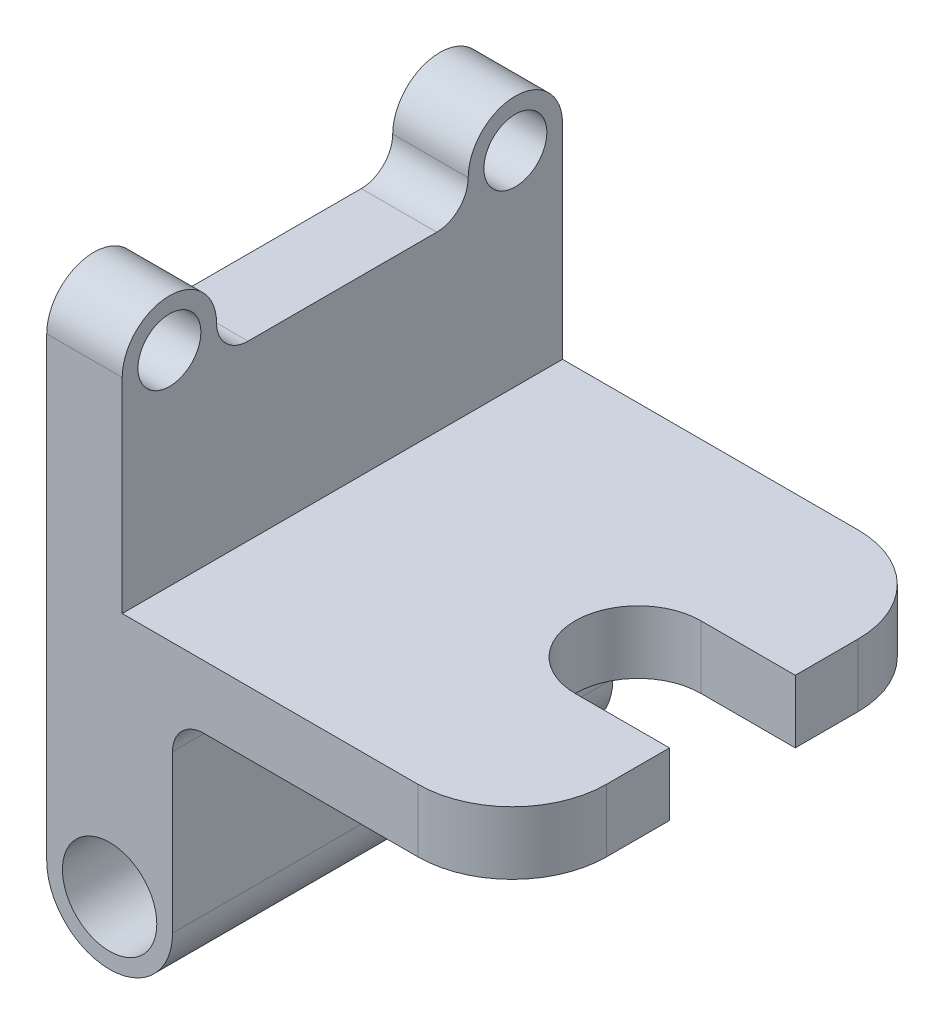
ISO-10303-21;
HEADER;
FILE_DESCRIPTION(('STEP AP214'),'2;1');
FILE_NAME('part.step','',(''),(''),'','','');
FILE_SCHEMA(('AUTOMOTIVE_DESIGN { 1 0 10303 214 1 1 1 1 }'));
ENDSEC;
DATA;
#1=APPLICATION_CONTEXT('core data for automotive mechanical design processes');
#2=APPLICATION_PROTOCOL_DEFINITION('international standard','automotive_design',2000,#1);
#3=PRODUCT_CONTEXT('',#1,'mechanical');
#4=PRODUCT('Part','Part','',(#3));
#5=PRODUCT_RELATED_PRODUCT_CATEGORY('part','',(#4));
#6=PRODUCT_DEFINITION_FORMATION('','',#4);
#7=PRODUCT_DEFINITION_CONTEXT('part definition',#1,'design');
#8=PRODUCT_DEFINITION('design','',#6,#7);
#9=PRODUCT_DEFINITION_SHAPE('','',#8);
#10=(LENGTH_UNIT() NAMED_UNIT(*) SI_UNIT(.MILLI.,.METRE.));
#11=(NAMED_UNIT(*) PLANE_ANGLE_UNIT() SI_UNIT($,.RADIAN.));
#12=(NAMED_UNIT(*) SI_UNIT($,.STERADIAN.) SOLID_ANGLE_UNIT());
#13=UNCERTAINTY_MEASURE_WITH_UNIT(LENGTH_MEASURE(1.E-05),#10,'distance_accuracy_value','');
#14=(GEOMETRIC_REPRESENTATION_CONTEXT(3) GLOBAL_UNCERTAINTY_ASSIGNED_CONTEXT((#13)) GLOBAL_UNIT_ASSIGNED_CONTEXT((#10,
#11,#12)) REPRESENTATION_CONTEXT('',''));
#15=CARTESIAN_POINT('',(0.,0.,0.));
#16=DIRECTION('',(0.,0.,1.));
#17=DIRECTION('',(1.,0.,0.));
#18=AXIS2_PLACEMENT_3D('',#15,#16,#17);
#19=CARTESIAN_POINT('',(0.,5.,35.));
#20=DIRECTION('',(0.,0.,-1.));
#21=DIRECTION('',(-1.,0.,0.));
#22=AXIS2_PLACEMENT_3D('',#19,#20,#21);
#23=PLANE('',#22);
#24=DIRECTION('',(0.,1.,0.));
#25=VECTOR('',#24,1.);
#26=CARTESIAN_POINT('',(-12.,-5.,35.));
#27=LINE('',#26,#25);
#28=CARTESIAN_POINT('',(-12.,-35.,35.));
#29=VERTEX_POINT('',#28);
#30=CARTESIAN_POINT('',(-12.,37.5,35.));
#31=VERTEX_POINT('',#30);
#32=EDGE_CURVE('E175',#29,#31,#27,.T.);
#33=ORIENTED_EDGE('',*,*,#32,.F.);
#34=CARTESIAN_POINT('',(-2.,-35.,35.));
#35=DIRECTION('',(0.,0.,1.));
#36=DIRECTION('',(1.,0.,0.));
#37=AXIS2_PLACEMENT_3D('',#34,#35,#36);
#38=CIRCLE('',#37,10.);
#39=CARTESIAN_POINT('',(8.,-35.,35.));
#40=VERTEX_POINT('',#39);
#41=EDGE_CURVE('E180',#29,#40,#38,.T.);
#42=ORIENTED_EDGE('',*,*,#41,.T.);
#43=DIRECTION('',(0.,1.,0.));
#44=VECTOR('',#43,1.);
#45=CARTESIAN_POINT('',(8.,-5.,35.));
#46=LINE('',#45,#44);
#47=CARTESIAN_POINT('',(8.,-10.,35.));
#48=VERTEX_POINT('',#47);
#49=EDGE_CURVE('E193',#40,#48,#46,.T.);
#50=ORIENTED_EDGE('',*,*,#49,.T.);
#51=CARTESIAN_POINT('',(13.,-10.,35.));
#52=DIRECTION('',(0.,0.,-1.));
#53=DIRECTION('',(-1.,0.,0.));
#54=AXIS2_PLACEMENT_3D('',#51,#52,#53);
#55=CIRCLE('',#54,5.);
#56=CARTESIAN_POINT('',(13.,-5.,35.));
#57=VERTEX_POINT('',#56);
#58=EDGE_CURVE('E11',#48,#57,#55,.T.);
#59=ORIENTED_EDGE('',*,*,#58,.T.);
#60=DIRECTION('',(1.,0.,0.));
#61=VECTOR('',#60,1.);
#62=CARTESIAN_POINT('',(0.,-5.,35.));
#63=LINE('',#62,#61);
#64=CARTESIAN_POINT('',(47.,-5.,35.));
#65=VERTEX_POINT('',#64);
#66=EDGE_CURVE('E246',#57,#65,#63,.T.);
#67=ORIENTED_EDGE('',*,*,#66,.T.);
#68=DIRECTION('',(0.,-1.,0.));
#69=VECTOR('',#68,1.);
#70=CARTESIAN_POINT('',(47.,5.,35.));
#71=LINE('',#70,#69);
#72=CARTESIAN_POINT('',(47.,5.,35.));
#73=VERTEX_POINT('',#72);
#74=EDGE_CURVE('E306',#73,#65,#71,.T.);
#75=ORIENTED_EDGE('',*,*,#74,.F.);
#76=DIRECTION('',(1.,0.,0.));
#77=VECTOR('',#76,1.);
#78=CARTESIAN_POINT('',(0.,5.,35.));
#79=LINE('',#78,#77);
#80=CARTESIAN_POINT('',(0.,5.,35.));
#81=VERTEX_POINT('',#80);
#82=EDGE_CURVE('E253',#81,#73,#79,.T.);
#83=ORIENTED_EDGE('',*,*,#82,.F.);
#84=DIRECTION('',(0.,1.,0.));
#85=VECTOR('',#84,1.);
#86=CARTESIAN_POINT('',(0.,5.,35.));
#87=LINE('',#86,#85);
#88=CARTESIAN_POINT('',(0.,37.5,35.));
#89=VERTEX_POINT('',#88);
#90=EDGE_CURVE('E214',#81,#89,#87,.T.);
#91=ORIENTED_EDGE('',*,*,#90,.T.);
#92=DIRECTION('',(1.,0.,0.));
#93=VECTOR('',#92,1.);
#94=CARTESIAN_POINT('',(-12.,37.5,35.));
#95=LINE('',#94,#93);
#96=EDGE_CURVE('E182',#31,#89,#95,.T.);
#97=ORIENTED_EDGE('',*,*,#96,.F.);
#98=EDGE_LOOP('',(#33,#42,#50,#59,#67,#75,#83,#91,#97));
#99=FACE_BOUND('',#98,.T.);
#100=CARTESIAN_POINT('',(-2.,-35.,35.));
#101=DIRECTION('',(0.,0.,1.));
#102=DIRECTION('',(1.,0.,0.));
#103=AXIS2_PLACEMENT_3D('',#100,#101,#102);
#104=CIRCLE('',#103,7.5);
#105=CARTESIAN_POINT('',(5.5,-35.,35.));
#106=VERTEX_POINT('',#105);
#107=EDGE_CURVE('E657',#106,#106,#104,.T.);
#108=ORIENTED_EDGE('',*,*,#107,.F.);
#109=EDGE_LOOP('',(#108));
#110=FACE_BOUND('',#109,.T.);
#111=ADVANCED_FACE('F44',(#99,#110),#23,.F.);
#112=CARTESIAN_POINT('',(47.,5.,20.));
#113=DIRECTION('',(0.,-1.,0.));
#114=DIRECTION('',(0.,0.,-1.));
#115=AXIS2_PLACEMENT_3D('',#112,#113,#114);
#116=CYLINDRICAL_SURFACE('',#115,15.);
#117=CARTESIAN_POINT('',(47.,-5.,20.));
#118=DIRECTION('',(0.,1.,0.));
#119=DIRECTION('',(0.,0.,1.));
#120=AXIS2_PLACEMENT_3D('',#117,#118,#119);
#121=CIRCLE('',#120,15.);
#122=CARTESIAN_POINT('',(62.,-5.,20.));
#123=VERTEX_POINT('',#122);
#124=EDGE_CURVE('E272',#65,#123,#121,.T.);
#125=ORIENTED_EDGE('',*,*,#124,.T.);
#126=DIRECTION('',(0.,-1.,0.));
#127=VECTOR('',#126,1.);
#128=CARTESIAN_POINT('',(62.,5.,20.));
#129=LINE('',#128,#127);
#130=CARTESIAN_POINT('',(62.,5.,20.));
#131=VERTEX_POINT('',#130);
#132=EDGE_CURVE('E302',#131,#123,#129,.T.);
#133=ORIENTED_EDGE('',*,*,#132,.F.);
#134=CARTESIAN_POINT('',(47.,5.,20.));
#135=DIRECTION('',(0.,1.,0.));
#136=DIRECTION('',(0.,0.,1.));
#137=AXIS2_PLACEMENT_3D('',#134,#135,#136);
#138=CIRCLE('',#137,15.);
#139=EDGE_CURVE('E255',#73,#131,#138,.T.);
#140=ORIENTED_EDGE('',*,*,#139,.F.);
#141=ORIENTED_EDGE('',*,*,#74,.T.);
#142=EDGE_LOOP('',(#125,#133,#140,#141));
#143=FACE_BOUND('',#142,.T.);
#144=ADVANCED_FACE('F371',(#143),#116,.T.);
#145=CARTESIAN_POINT('',(62.,5.,10.));
#146=DIRECTION('',(-1.,0.,0.));
#147=DIRECTION('',(0.,0.,1.));
#148=AXIS2_PLACEMENT_3D('',#145,#146,#147);
#149=PLANE('',#148);
#150=DIRECTION('',(0.,0.,-1.));
#151=VECTOR('',#150,1.);
#152=CARTESIAN_POINT('',(62.,-5.,10.));
#153=LINE('',#152,#151);
#154=CARTESIAN_POINT('',(62.,-5.,10.));
#155=VERTEX_POINT('',#154);
#156=EDGE_CURVE('E274',#123,#155,#153,.T.);
#157=ORIENTED_EDGE('',*,*,#156,.T.);
#158=DIRECTION('',(0.,-1.,0.));
#159=VECTOR('',#158,1.);
#160=CARTESIAN_POINT('',(62.,5.,10.));
#161=LINE('',#160,#159);
#162=CARTESIAN_POINT('',(62.,5.,10.));
#163=VERTEX_POINT('',#162);
#164=EDGE_CURVE('E301',#163,#155,#161,.T.);
#165=ORIENTED_EDGE('',*,*,#164,.F.);
#166=DIRECTION('',(0.,0.,-1.));
#167=VECTOR('',#166,1.);
#168=CARTESIAN_POINT('',(62.,5.,10.));
#169=LINE('',#168,#167);
#170=EDGE_CURVE('E258',#131,#163,#169,.T.);
#171=ORIENTED_EDGE('',*,*,#170,.F.);
#172=ORIENTED_EDGE('',*,*,#132,.T.);
#173=EDGE_LOOP('',(#157,#165,#171,#172));
#174=FACE_BOUND('',#173,.T.);
#175=ADVANCED_FACE('F370',(#174),#149,.F.);
#176=CARTESIAN_POINT('',(47.,5.,10.));
#177=DIRECTION('',(0.,0.,1.));
#178=DIRECTION('',(1.,0.,0.));
#179=AXIS2_PLACEMENT_3D('',#176,#177,#178);
#180=PLANE('',#179);
#181=DIRECTION('',(-1.,0.,0.));
#182=VECTOR('',#181,1.);
#183=CARTESIAN_POINT('',(47.,-5.,10.));
#184=LINE('',#183,#182);
#185=CARTESIAN_POINT('',(47.,-5.,10.));
#186=VERTEX_POINT('',#185);
#187=EDGE_CURVE('E280',#155,#186,#184,.T.);
#188=ORIENTED_EDGE('',*,*,#187,.T.);
#189=DIRECTION('',(0.,-1.,0.));
#190=VECTOR('',#189,1.);
#191=CARTESIAN_POINT('',(47.,5.,10.));
#192=LINE('',#191,#190);
#193=CARTESIAN_POINT('',(47.,5.,10.));
#194=VERTEX_POINT('',#193);
#195=EDGE_CURVE('E298',#194,#186,#192,.T.);
#196=ORIENTED_EDGE('',*,*,#195,.F.);
#197=DIRECTION('',(-1.,0.,0.));
#198=VECTOR('',#197,1.);
#199=CARTESIAN_POINT('',(47.,5.,10.));
#200=LINE('',#199,#198);
#201=EDGE_CURVE('E256',#163,#194,#200,.T.);
#202=ORIENTED_EDGE('',*,*,#201,.F.);
#203=ORIENTED_EDGE('',*,*,#164,.T.);
#204=EDGE_LOOP('',(#188,#196,#202,#203));
#205=FACE_BOUND('',#204,.T.);
#206=ADVANCED_FACE('F362',(#205),#180,.F.);
#207=CARTESIAN_POINT('',(47.,5.,0.));
#208=DIRECTION('',(0.,-1.,0.));
#209=DIRECTION('',(0.,0.,-1.));
#210=AXIS2_PLACEMENT_3D('',#207,#208,#209);
#211=CYLINDRICAL_SURFACE('',#210,10.);
#212=CARTESIAN_POINT('',(47.,-5.,0.));
#213=DIRECTION('',(0.,-1.,0.));
#214=DIRECTION('',(0.,0.,1.));
#215=AXIS2_PLACEMENT_3D('',#212,#213,#214);
#216=CIRCLE('',#215,10.);
#217=CARTESIAN_POINT('',(47.,-5.,-10.));
#218=VERTEX_POINT('',#217);
#219=EDGE_CURVE('E276',#186,#218,#216,.T.);
#220=ORIENTED_EDGE('',*,*,#219,.T.);
#221=DIRECTION('',(0.,-1.,0.));
#222=VECTOR('',#221,1.);
#223=CARTESIAN_POINT('',(47.,5.,-10.));
#224=LINE('',#223,#222);
#225=CARTESIAN_POINT('',(47.,5.,-10.));
#226=VERTEX_POINT('',#225);
#227=EDGE_CURVE('E296',#226,#218,#224,.T.);
#228=ORIENTED_EDGE('',*,*,#227,.F.);
#229=CARTESIAN_POINT('',(47.,5.,0.));
#230=DIRECTION('',(0.,-1.,0.));
#231=DIRECTION('',(0.,0.,1.));
#232=AXIS2_PLACEMENT_3D('',#229,#230,#231);
#233=CIRCLE('',#232,10.);
#234=EDGE_CURVE('E257',#194,#226,#233,.T.);
#235=ORIENTED_EDGE('',*,*,#234,.F.);
#236=ORIENTED_EDGE('',*,*,#195,.T.);
#237=EDGE_LOOP('',(#220,#228,#235,#236));
#238=FACE_BOUND('',#237,.T.);
#239=ADVANCED_FACE('F356',(#238),#211,.F.);
#240=CARTESIAN_POINT('',(47.,5.,-10.));
#241=DIRECTION('',(0.,0.,-1.));
#242=DIRECTION('',(-1.,0.,0.));
#243=AXIS2_PLACEMENT_3D('',#240,#241,#242);
#244=PLANE('',#243);
#245=DIRECTION('',(1.,0.,0.));
#246=VECTOR('',#245,1.);
#247=CARTESIAN_POINT('',(47.,-5.,-10.));
#248=LINE('',#247,#246);
#249=CARTESIAN_POINT('',(62.,-5.,-10.));
#250=VERTEX_POINT('',#249);
#251=EDGE_CURVE('E281',#218,#250,#248,.T.);
#252=ORIENTED_EDGE('',*,*,#251,.T.);
#253=DIRECTION('',(0.,-1.,0.));
#254=VECTOR('',#253,1.);
#255=CARTESIAN_POINT('',(62.,5.,-10.));
#256=LINE('',#255,#254);
#257=CARTESIAN_POINT('',(62.,5.,-10.));
#258=VERTEX_POINT('',#257);
#259=EDGE_CURVE('E291',#258,#250,#256,.T.);
#260=ORIENTED_EDGE('',*,*,#259,.F.);
#261=DIRECTION('',(1.,0.,0.));
#262=VECTOR('',#261,1.);
#263=CARTESIAN_POINT('',(47.,5.,-10.));
#264=LINE('',#263,#262);
#265=EDGE_CURVE('E265',#226,#258,#264,.T.);
#266=ORIENTED_EDGE('',*,*,#265,.F.);
#267=ORIENTED_EDGE('',*,*,#227,.T.);
#268=EDGE_LOOP('',(#252,#260,#266,#267));
#269=FACE_BOUND('',#268,.T.);
#270=ADVANCED_FACE('F354',(#269),#244,.F.);
#271=CARTESIAN_POINT('',(62.,5.,-20.));
#272=DIRECTION('',(-1.,0.,0.));
#273=DIRECTION('',(0.,0.,1.));
#274=AXIS2_PLACEMENT_3D('',#271,#272,#273);
#275=PLANE('',#274);
#276=DIRECTION('',(0.,0.,-1.));
#277=VECTOR('',#276,1.);
#278=CARTESIAN_POINT('',(62.,-5.,-20.));
#279=LINE('',#278,#277);
#280=CARTESIAN_POINT('',(62.,-5.,-20.));
#281=VERTEX_POINT('',#280);
#282=EDGE_CURVE('E284',#250,#281,#279,.T.);
#283=ORIENTED_EDGE('',*,*,#282,.T.);
#284=DIRECTION('',(0.,-1.,0.));
#285=VECTOR('',#284,1.);
#286=CARTESIAN_POINT('',(62.,5.,-20.));
#287=LINE('',#286,#285);
#288=CARTESIAN_POINT('',(62.,5.,-20.));
#289=VERTEX_POINT('',#288);
#290=EDGE_CURVE('E287',#289,#281,#287,.T.);
#291=ORIENTED_EDGE('',*,*,#290,.F.);
#292=DIRECTION('',(0.,0.,-1.));
#293=VECTOR('',#292,1.);
#294=CARTESIAN_POINT('',(62.,5.,-20.));
#295=LINE('',#294,#293);
#296=EDGE_CURVE('E262',#258,#289,#295,.T.);
#297=ORIENTED_EDGE('',*,*,#296,.F.);
#298=ORIENTED_EDGE('',*,*,#259,.T.);
#299=EDGE_LOOP('',(#283,#291,#297,#298));
#300=FACE_BOUND('',#299,.T.);
#301=ADVANCED_FACE('F346',(#300),#275,.F.);
#302=CARTESIAN_POINT('',(47.,5.,-20.));
#303=DIRECTION('',(0.,-1.,0.));
#304=DIRECTION('',(0.,0.,-1.));
#305=AXIS2_PLACEMENT_3D('',#302,#303,#304);
#306=CYLINDRICAL_SURFACE('',#305,15.);
#307=CARTESIAN_POINT('',(47.,-5.,-20.));
#308=DIRECTION('',(0.,1.,0.));
#309=DIRECTION('',(0.,0.,-1.));
#310=AXIS2_PLACEMENT_3D('',#307,#308,#309);
#311=CIRCLE('',#310,15.);
#312=CARTESIAN_POINT('',(47.,-5.,-35.));
#313=VERTEX_POINT('',#312);
#314=EDGE_CURVE('E285',#281,#313,#311,.T.);
#315=ORIENTED_EDGE('',*,*,#314,.T.);
#316=DIRECTION('',(0.,-1.,0.));
#317=VECTOR('',#316,1.);
#318=CARTESIAN_POINT('',(47.,5.,-35.));
#319=LINE('',#318,#317);
#320=CARTESIAN_POINT('',(47.,5.,-35.));
#321=VERTEX_POINT('',#320);
#322=EDGE_CURVE('E271',#321,#313,#319,.T.);
#323=ORIENTED_EDGE('',*,*,#322,.F.);
#324=CARTESIAN_POINT('',(47.,5.,-20.));
#325=DIRECTION('',(0.,1.,0.));
#326=DIRECTION('',(0.,0.,-1.));
#327=AXIS2_PLACEMENT_3D('',#324,#325,#326);
#328=CIRCLE('',#327,15.);
#329=EDGE_CURVE('E266',#289,#321,#328,.T.);
#330=ORIENTED_EDGE('',*,*,#329,.F.);
#331=ORIENTED_EDGE('',*,*,#290,.T.);
#332=EDGE_LOOP('',(#315,#323,#330,#331));
#333=FACE_BOUND('',#332,.T.);
#334=ADVANCED_FACE('F341',(#333),#306,.T.);
#335=CARTESIAN_POINT('',(0.,5.,-35.));
#336=DIRECTION('',(0.,0.,1.));
#337=DIRECTION('',(1.,0.,0.));
#338=AXIS2_PLACEMENT_3D('',#335,#336,#337);
#339=PLANE('',#338);
#340=DIRECTION('',(-1.,0.,0.));
#341=VECTOR('',#340,1.);
#342=CARTESIAN_POINT('',(0.,-5.,-35.));
#343=LINE('',#342,#341);
#344=CARTESIAN_POINT('',(13.,-5.,-35.));
#345=VERTEX_POINT('',#344);
#346=EDGE_CURVE('E252',#313,#345,#343,.T.);
#347=ORIENTED_EDGE('',*,*,#346,.T.);
#348=CARTESIAN_POINT('',(13.,-10.,-35.));
#349=DIRECTION('',(0.,0.,1.));
#350=DIRECTION('',(1.,0.,0.));
#351=AXIS2_PLACEMENT_3D('',#348,#349,#350);
#352=CIRCLE('',#351,5.);
#353=CARTESIAN_POINT('',(8.,-10.,-35.));
#354=VERTEX_POINT('',#353);
#355=EDGE_CURVE('E52',#345,#354,#352,.T.);
#356=ORIENTED_EDGE('',*,*,#355,.T.);
#357=DIRECTION('',(0.,1.,0.));
#358=VECTOR('',#357,1.);
#359=CARTESIAN_POINT('',(8.,-5.,-35.));
#360=LINE('',#359,#358);
#361=CARTESIAN_POINT('',(8.,-35.,-35.));
#362=VERTEX_POINT('',#361);
#363=EDGE_CURVE('E192',#362,#354,#360,.T.);
#364=ORIENTED_EDGE('',*,*,#363,.F.);
#365=CARTESIAN_POINT('',(-2.,-35.,-35.));
#366=DIRECTION('',(0.,0.,1.));
#367=DIRECTION('',(1.,0.,0.));
#368=AXIS2_PLACEMENT_3D('',#365,#366,#367);
#369=CIRCLE('',#368,10.);
#370=CARTESIAN_POINT('',(-12.,-35.,-35.));
#371=VERTEX_POINT('',#370);
#372=EDGE_CURVE('E660',#371,#362,#369,.T.);
#373=ORIENTED_EDGE('',*,*,#372,.F.);
#374=DIRECTION('',(0.,-1.,0.));
#375=VECTOR('',#374,1.);
#376=CARTESIAN_POINT('',(-12.,5.,-35.));
#377=LINE('',#376,#375);
#378=CARTESIAN_POINT('',(-12.,37.5,-35.));
#379=VERTEX_POINT('',#378);
#380=EDGE_CURVE('E186',#379,#371,#377,.T.);
#381=ORIENTED_EDGE('',*,*,#380,.F.);
#382=DIRECTION('',(1.,0.,0.));
#383=VECTOR('',#382,1.);
#384=CARTESIAN_POINT('',(-12.,37.5,-35.));
#385=LINE('',#384,#383);
#386=CARTESIAN_POINT('',(0.,37.5,-35.));
#387=VERTEX_POINT('',#386);
#388=EDGE_CURVE('E226',#379,#387,#385,.T.);
#389=ORIENTED_EDGE('',*,*,#388,.T.);
#390=DIRECTION('',(0.,-1.,0.));
#391=VECTOR('',#390,1.);
#392=CARTESIAN_POINT('',(0.,5.,-35.));
#393=LINE('',#392,#391);
#394=CARTESIAN_POINT('',(0.,5.,-35.));
#395=VERTEX_POINT('',#394);
#396=EDGE_CURVE('E217',#387,#395,#393,.T.);
#397=ORIENTED_EDGE('',*,*,#396,.T.);
#398=DIRECTION('',(-1.,0.,0.));
#399=VECTOR('',#398,1.);
#400=CARTESIAN_POINT('',(0.,5.,-35.));
#401=LINE('',#400,#399);
#402=EDGE_CURVE('E268',#321,#395,#401,.T.);
#403=ORIENTED_EDGE('',*,*,#402,.F.);
#404=ORIENTED_EDGE('',*,*,#322,.T.);
#405=EDGE_LOOP('',(#347,#356,#364,#373,#381,#389,#397,#403,#404));
#406=FACE_BOUND('',#405,.T.);
#407=CARTESIAN_POINT('',(-2.,-35.,-35.));
#408=DIRECTION('',(0.,0.,1.));
#409=DIRECTION('',(1.,0.,0.));
#410=AXIS2_PLACEMENT_3D('',#407,#408,#409);
#411=CIRCLE('',#410,7.5);
#412=CARTESIAN_POINT('',(5.5,-35.,-35.));
#413=VERTEX_POINT('',#412);
#414=EDGE_CURVE('E665',#413,#413,#411,.T.);
#415=ORIENTED_EDGE('',*,*,#414,.T.);
#416=EDGE_LOOP('',(#415));
#417=FACE_BOUND('',#416,.T.);
#418=ADVANCED_FACE('F336',(#406,#417),#339,.F.);
#419=CARTESIAN_POINT('',(47.,5.,20.));
#420=DIRECTION('',(0.,1.,0.));
#421=DIRECTION('',(0.,0.,1.));
#422=AXIS2_PLACEMENT_3D('',#419,#420,#421);
#423=PLANE('',#422);
#424=DIRECTION('',(0.,0.,1.));
#425=VECTOR('',#424,1.);
#426=CARTESIAN_POINT('',(0.,5.,-35.));
#427=LINE('',#426,#425);
#428=EDGE_CURVE('E250',#395,#81,#427,.T.);
#429=ORIENTED_EDGE('',*,*,#428,.T.);
#430=ORIENTED_EDGE('',*,*,#82,.T.);
#431=ORIENTED_EDGE('',*,*,#139,.T.);
#432=ORIENTED_EDGE('',*,*,#170,.T.);
#433=ORIENTED_EDGE('',*,*,#201,.T.);
#434=ORIENTED_EDGE('',*,*,#234,.T.);
#435=ORIENTED_EDGE('',*,*,#265,.T.);
#436=ORIENTED_EDGE('',*,*,#296,.T.);
#437=ORIENTED_EDGE('',*,*,#329,.T.);
#438=ORIENTED_EDGE('',*,*,#402,.T.);
#439=EDGE_LOOP('',(#429,#430,#431,#432,#433,#434,#435,#436,#437,#438));
#440=FACE_BOUND('',#439,.T.);
#441=ADVANCED_FACE('F419',(#440),#423,.T.);
#442=CARTESIAN_POINT('',(47.,-5.,20.));
#443=DIRECTION('',(0.,1.,0.));
#444=DIRECTION('',(0.,0.,1.));
#445=AXIS2_PLACEMENT_3D('',#442,#443,#444);
#446=PLANE('',#445);
#447=ORIENTED_EDGE('',*,*,#66,.F.);
#448=DIRECTION('',(0.,0.,-1.));
#449=VECTOR('',#448,1.);
#450=CARTESIAN_POINT('',(13.,-5.,-35.));
#451=LINE('',#450,#449);
#452=EDGE_CURVE('E322',#57,#345,#451,.T.);
#453=ORIENTED_EDGE('',*,*,#452,.T.);
#454=ORIENTED_EDGE('',*,*,#346,.F.);
#455=ORIENTED_EDGE('',*,*,#314,.F.);
#456=ORIENTED_EDGE('',*,*,#282,.F.);
#457=ORIENTED_EDGE('',*,*,#251,.F.);
#458=ORIENTED_EDGE('',*,*,#219,.F.);
#459=ORIENTED_EDGE('',*,*,#187,.F.);
#460=ORIENTED_EDGE('',*,*,#156,.F.);
#461=ORIENTED_EDGE('',*,*,#124,.F.);
#462=EDGE_LOOP('',(#447,#453,#454,#455,#456,#457,#458,#459,#460,#461));
#463=FACE_BOUND('',#462,.T.);
#464=ADVANCED_FACE('F332',(#463),#446,.F.);
#465=CARTESIAN_POINT('',(-12.,37.5,27.5));
#466=DIRECTION('',(-1.,0.,0.));
#467=DIRECTION('',(0.,0.,1.));
#468=AXIS2_PLACEMENT_3D('',#465,#466,#467);
#469=PLANE('',#468);
#470=CARTESIAN_POINT('',(-12.,37.5,-27.5));
#471=DIRECTION('',(-1.,0.,0.));
#472=DIRECTION('',(0.,0.,1.));
#473=AXIS2_PLACEMENT_3D('',#470,#471,#472);
#474=CIRCLE('',#473,5.);
#475=CARTESIAN_POINT('',(-12.,37.5,-22.5));
#476=VERTEX_POINT('',#475);
#477=EDGE_CURVE('E215',#476,#476,#474,.T.);
#478=ORIENTED_EDGE('',*,*,#477,.F.);
#479=EDGE_LOOP('',(#478));
#480=FACE_BOUND('',#479,.T.);
#481=ORIENTED_EDGE('',*,*,#380,.T.);
#482=DIRECTION('',(0.,0.,-1.));
#483=VECTOR('',#482,1.);
#484=CARTESIAN_POINT('',(-12.,-35.,35.));
#485=LINE('',#484,#483);
#486=EDGE_CURVE('E194',#29,#371,#485,.T.);
#487=ORIENTED_EDGE('',*,*,#486,.F.);
#488=ORIENTED_EDGE('',*,*,#32,.T.);
#489=CARTESIAN_POINT('',(-12.,37.5,27.5));
#490=DIRECTION('',(-1.,0.,0.));
#491=DIRECTION('',(0.,0.,1.));
#492=AXIS2_PLACEMENT_3D('',#489,#490,#491);
#493=CIRCLE('',#492,7.5);
#494=CARTESIAN_POINT('',(-12.,37.5,20.));
#495=VERTEX_POINT('',#494);
#496=EDGE_CURVE('E183',#31,#495,#493,.T.);
#497=ORIENTED_EDGE('',*,*,#496,.T.);
#498=CARTESIAN_POINT('',(-12.,37.5,15.));
#499=DIRECTION('',(-1.,0.,0.));
#500=DIRECTION('',(0.,0.,1.));
#501=AXIS2_PLACEMENT_3D('',#498,#499,#500);
#502=CIRCLE('',#501,5.);
#503=CARTESIAN_POINT('',(-12.,32.5,15.));
#504=VERTEX_POINT('',#503);
#505=EDGE_CURVE('E318',#495,#504,#502,.F.);
#506=ORIENTED_EDGE('',*,*,#505,.T.);
#507=DIRECTION('',(0.,0.,-1.));
#508=VECTOR('',#507,1.);
#509=CARTESIAN_POINT('',(-12.,32.5,-20.));
#510=LINE('',#509,#508);
#511=CARTESIAN_POINT('',(-12.,32.5,-15.));
#512=VERTEX_POINT('',#511);
#513=EDGE_CURVE('E222',#504,#512,#510,.T.);
#514=ORIENTED_EDGE('',*,*,#513,.T.);
#515=CARTESIAN_POINT('',(-12.,37.5,-15.));
#516=DIRECTION('',(-1.,0.,0.));
#517=DIRECTION('',(0.,0.,1.));
#518=AXIS2_PLACEMENT_3D('',#515,#516,#517);
#519=CIRCLE('',#518,5.);
#520=CARTESIAN_POINT('',(-12.,37.5,-20.));
#521=VERTEX_POINT('',#520);
#522=EDGE_CURVE('E325',#512,#521,#519,.F.);
#523=ORIENTED_EDGE('',*,*,#522,.T.);
#524=CARTESIAN_POINT('',(-12.,37.5,-27.5));
#525=DIRECTION('',(-1.,0.,0.));
#526=DIRECTION('',(0.,0.,-1.));
#527=AXIS2_PLACEMENT_3D('',#524,#525,#526);
#528=CIRCLE('',#527,7.5);
#529=EDGE_CURVE('E221',#521,#379,#528,.T.);
#530=ORIENTED_EDGE('',*,*,#529,.T.);
#531=EDGE_LOOP('',(#481,#487,#488,#497,#506,#514,#523,#530));
#532=FACE_BOUND('',#531,.T.);
#533=CARTESIAN_POINT('',(-12.,37.5,27.5));
#534=DIRECTION('',(-1.,0.,0.));
#535=DIRECTION('',(0.,0.,1.));
#536=AXIS2_PLACEMENT_3D('',#533,#534,#535);
#537=CIRCLE('',#536,5.);
#538=CARTESIAN_POINT('',(-12.,37.5,32.5));
#539=VERTEX_POINT('',#538);
#540=EDGE_CURVE('E204',#539,#539,#537,.T.);
#541=ORIENTED_EDGE('',*,*,#540,.F.);
#542=EDGE_LOOP('',(#541));
#543=FACE_BOUND('',#542,.T.);
#544=ADVANCED_FACE('F197',(#480,#532,#543),#469,.T.);
#545=CARTESIAN_POINT('',(0.,37.5,27.5));
#546=DIRECTION('',(-1.,0.,0.));
#547=DIRECTION('',(0.,0.,1.));
#548=AXIS2_PLACEMENT_3D('',#545,#546,#547);
#549=PLANE('',#548);
#550=ORIENTED_EDGE('',*,*,#428,.F.);
#551=ORIENTED_EDGE('',*,*,#396,.F.);
#552=CARTESIAN_POINT('',(0.,37.5,-27.5));
#553=DIRECTION('',(-1.,0.,0.));
#554=DIRECTION('',(0.,0.,-1.));
#555=AXIS2_PLACEMENT_3D('',#552,#553,#554);
#556=CIRCLE('',#555,7.5);
#557=CARTESIAN_POINT('',(0.,37.5,-20.));
#558=VERTEX_POINT('',#557);
#559=EDGE_CURVE('E233',#558,#387,#556,.T.);
#560=ORIENTED_EDGE('',*,*,#559,.F.);
#561=CARTESIAN_POINT('',(0.,37.5,-15.));
#562=DIRECTION('',(-1.,0.,0.));
#563=DIRECTION('',(0.,0.,1.));
#564=AXIS2_PLACEMENT_3D('',#561,#562,#563);
#565=CIRCLE('',#564,5.);
#566=CARTESIAN_POINT('',(0.,32.5,-15.));
#567=VERTEX_POINT('',#566);
#568=EDGE_CURVE('E319',#558,#567,#565,.T.);
#569=ORIENTED_EDGE('',*,*,#568,.T.);
#570=DIRECTION('',(0.,0.,-1.));
#571=VECTOR('',#570,1.);
#572=CARTESIAN_POINT('',(0.,32.5,-20.));
#573=LINE('',#572,#571);
#574=CARTESIAN_POINT('',(0.,32.5,15.));
#575=VERTEX_POINT('',#574);
#576=EDGE_CURVE('E234',#575,#567,#573,.T.);
#577=ORIENTED_EDGE('',*,*,#576,.F.);
#578=CARTESIAN_POINT('',(0.,37.5,15.));
#579=DIRECTION('',(-1.,0.,0.));
#580=DIRECTION('',(0.,0.,1.));
#581=AXIS2_PLACEMENT_3D('',#578,#579,#580);
#582=CIRCLE('',#581,5.);
#583=CARTESIAN_POINT('',(0.,37.5,20.));
#584=VERTEX_POINT('',#583);
#585=EDGE_CURVE('E316',#575,#584,#582,.T.);
#586=ORIENTED_EDGE('',*,*,#585,.T.);
#587=CARTESIAN_POINT('',(0.,37.5,27.5));
#588=DIRECTION('',(-1.,0.,0.));
#589=DIRECTION('',(0.,0.,1.));
#590=AXIS2_PLACEMENT_3D('',#587,#588,#589);
#591=CIRCLE('',#590,7.5);
#592=EDGE_CURVE('E229',#89,#584,#591,.T.);
#593=ORIENTED_EDGE('',*,*,#592,.F.);
#594=ORIENTED_EDGE('',*,*,#90,.F.);
#595=EDGE_LOOP('',(#550,#551,#560,#569,#577,#586,#593,#594));
#596=FACE_BOUND('',#595,.T.);
#597=CARTESIAN_POINT('',(0.,37.5,-27.5));
#598=DIRECTION('',(-1.,0.,0.));
#599=DIRECTION('',(0.,0.,1.));
#600=AXIS2_PLACEMENT_3D('',#597,#598,#599);
#601=CIRCLE('',#600,5.);
#602=CARTESIAN_POINT('',(0.,37.5,-22.5));
#603=VERTEX_POINT('',#602);
#604=EDGE_CURVE('E209',#603,#603,#601,.T.);
#605=ORIENTED_EDGE('',*,*,#604,.T.);
#606=EDGE_LOOP('',(#605));
#607=FACE_BOUND('',#606,.T.);
#608=CARTESIAN_POINT('',(0.,37.5,27.5));
#609=DIRECTION('',(-1.,0.,0.));
#610=DIRECTION('',(0.,0.,1.));
#611=AXIS2_PLACEMENT_3D('',#608,#609,#610);
#612=CIRCLE('',#611,5.);
#613=CARTESIAN_POINT('',(0.,37.5,32.5));
#614=VERTEX_POINT('',#613);
#615=EDGE_CURVE('E203',#614,#614,#612,.T.);
#616=ORIENTED_EDGE('',*,*,#615,.T.);
#617=EDGE_LOOP('',(#616));
#618=FACE_BOUND('',#617,.T.);
#619=ADVANCED_FACE('F418',(#596,#607,#618),#549,.F.);
#620=CARTESIAN_POINT('',(-12.,37.5,27.5));
#621=DIRECTION('',(1.,0.,0.));
#622=DIRECTION('',(0.,0.,-1.));
#623=AXIS2_PLACEMENT_3D('',#620,#621,#622);
#624=CYLINDRICAL_SURFACE('',#623,7.5);
#625=ORIENTED_EDGE('',*,*,#592,.T.);
#626=DIRECTION('',(1.,0.,0.));
#627=VECTOR('',#626,1.);
#628=CARTESIAN_POINT('',(-12.,37.5,20.));
#629=LINE('',#628,#627);
#630=EDGE_CURVE('E244',#495,#584,#629,.T.);
#631=ORIENTED_EDGE('',*,*,#630,.F.);
#632=ORIENTED_EDGE('',*,*,#496,.F.);
#633=ORIENTED_EDGE('',*,*,#96,.T.);
#634=EDGE_LOOP('',(#625,#631,#632,#633));
#635=FACE_BOUND('',#634,.T.);
#636=ADVANCED_FACE('F431',(#635),#624,.T.);
#637=CARTESIAN_POINT('',(-12.,32.5,-20.));
#638=DIRECTION('',(0.,-1.,0.));
#639=DIRECTION('',(0.,0.,-1.));
#640=AXIS2_PLACEMENT_3D('',#637,#638,#639);
#641=PLANE('',#640);
#642=ORIENTED_EDGE('',*,*,#513,.F.);
#643=DIRECTION('',(1.,0.,0.));
#644=VECTOR('',#643,1.);
#645=CARTESIAN_POINT('',(0.,32.5,15.));
#646=LINE('',#645,#644);
#647=EDGE_CURVE('E311',#504,#575,#646,.T.);
#648=ORIENTED_EDGE('',*,*,#647,.T.);
#649=ORIENTED_EDGE('',*,*,#576,.T.);
#650=DIRECTION('',(1.,0.,0.));
#651=VECTOR('',#650,1.);
#652=CARTESIAN_POINT('',(-12.,32.5,-15.));
#653=LINE('',#652,#651);
#654=EDGE_CURVE('E313',#567,#512,#653,.F.);
#655=ORIENTED_EDGE('',*,*,#654,.T.);
#656=EDGE_LOOP('',(#642,#648,#649,#655));
#657=FACE_BOUND('',#656,.T.);
#658=ADVANCED_FACE('F611',(#657),#641,.F.);
#659=CARTESIAN_POINT('',(-12.,37.5,-27.5));
#660=DIRECTION('',(1.,0.,0.));
#661=DIRECTION('',(0.,0.,-1.));
#662=AXIS2_PLACEMENT_3D('',#659,#660,#661);
#663=CYLINDRICAL_SURFACE('',#662,7.5);
#664=ORIENTED_EDGE('',*,*,#559,.T.);
#665=ORIENTED_EDGE('',*,*,#388,.F.);
#666=ORIENTED_EDGE('',*,*,#529,.F.);
#667=DIRECTION('',(1.,0.,0.));
#668=VECTOR('',#667,1.);
#669=CARTESIAN_POINT('',(-12.,37.5,-20.));
#670=LINE('',#669,#668);
#671=EDGE_CURVE('E238',#521,#558,#670,.T.);
#672=ORIENTED_EDGE('',*,*,#671,.T.);
#673=EDGE_LOOP('',(#664,#665,#666,#672));
#674=FACE_BOUND('',#673,.T.);
#675=ADVANCED_FACE('F411',(#674),#663,.T.);
#676=CARTESIAN_POINT('',(-12.,37.5,-27.5));
#677=DIRECTION('',(1.,0.,0.));
#678=DIRECTION('',(0.,0.,-1.));
#679=AXIS2_PLACEMENT_3D('',#676,#677,#678);
#680=CYLINDRICAL_SURFACE('',#679,5.);
#681=ORIENTED_EDGE('',*,*,#477,.T.);
#682=EDGE_LOOP('',(#681));
#683=FACE_BOUND('',#682,.T.);
#684=ORIENTED_EDGE('',*,*,#604,.F.);
#685=EDGE_LOOP('',(#684));
#686=FACE_BOUND('',#685,.T.);
#687=ADVANCED_FACE('F572',(#683,#686),#680,.F.);
#688=CARTESIAN_POINT('',(-12.,37.5,27.5));
#689=DIRECTION('',(1.,0.,0.));
#690=DIRECTION('',(0.,0.,-1.));
#691=AXIS2_PLACEMENT_3D('',#688,#689,#690);
#692=CYLINDRICAL_SURFACE('',#691,5.);
#693=ORIENTED_EDGE('',*,*,#540,.T.);
#694=EDGE_LOOP('',(#693));
#695=FACE_BOUND('',#694,.T.);
#696=ORIENTED_EDGE('',*,*,#615,.F.);
#697=EDGE_LOOP('',(#696));
#698=FACE_BOUND('',#697,.T.);
#699=ADVANCED_FACE('F399',(#695,#698),#692,.F.);
#700=CARTESIAN_POINT('',(-12.,37.5,15.));
#701=DIRECTION('',(-1.,0.,0.));
#702=DIRECTION('',(0.,0.,1.));
#703=AXIS2_PLACEMENT_3D('',#700,#701,#702);
#704=CYLINDRICAL_SURFACE('',#703,5.);
#705=ORIENTED_EDGE('',*,*,#505,.F.);
#706=ORIENTED_EDGE('',*,*,#630,.T.);
#707=ORIENTED_EDGE('',*,*,#585,.F.);
#708=ORIENTED_EDGE('',*,*,#647,.F.);
#709=EDGE_LOOP('',(#705,#706,#707,#708));
#710=FACE_BOUND('',#709,.T.);
#711=ADVANCED_FACE('F394',(#710),#704,.F.);
#712=CARTESIAN_POINT('',(-12.,37.5,-15.));
#713=DIRECTION('',(-1.,0.,0.));
#714=DIRECTION('',(0.,0.,1.));
#715=AXIS2_PLACEMENT_3D('',#712,#713,#714);
#716=CYLINDRICAL_SURFACE('',#715,5.);
#717=ORIENTED_EDGE('',*,*,#522,.F.);
#718=ORIENTED_EDGE('',*,*,#654,.F.);
#719=ORIENTED_EDGE('',*,*,#568,.F.);
#720=ORIENTED_EDGE('',*,*,#671,.F.);
#721=EDGE_LOOP('',(#717,#718,#719,#720));
#722=FACE_BOUND('',#721,.T.);
#723=ADVANCED_FACE('F395',(#722),#716,.F.);
#724=CARTESIAN_POINT('',(-2.,-35.,35.));
#725=DIRECTION('',(0.,0.,-1.));
#726=DIRECTION('',(-1.,0.,0.));
#727=AXIS2_PLACEMENT_3D('',#724,#725,#726);
#728=CYLINDRICAL_SURFACE('',#727,10.);
#729=ORIENTED_EDGE('',*,*,#372,.T.);
#730=DIRECTION('',(0.,0.,-1.));
#731=VECTOR('',#730,1.);
#732=CARTESIAN_POINT('',(8.,-35.,35.));
#733=LINE('',#732,#731);
#734=EDGE_CURVE('E195',#40,#362,#733,.T.);
#735=ORIENTED_EDGE('',*,*,#734,.F.);
#736=ORIENTED_EDGE('',*,*,#41,.F.);
#737=ORIENTED_EDGE('',*,*,#486,.T.);
#738=EDGE_LOOP('',(#729,#735,#736,#737));
#739=FACE_BOUND('',#738,.T.);
#740=ADVANCED_FACE('F190',(#739),#728,.T.);
#741=CARTESIAN_POINT('',(8.,-5.,35.));
#742=DIRECTION('',(-1.,0.,0.));
#743=DIRECTION('',(0.,-1.,0.));
#744=AXIS2_PLACEMENT_3D('',#741,#742,#743);
#745=PLANE('',#744);
#746=ORIENTED_EDGE('',*,*,#363,.T.);
#747=DIRECTION('',(0.,0.,-1.));
#748=VECTOR('',#747,1.);
#749=CARTESIAN_POINT('',(8.,-10.,35.));
#750=LINE('',#749,#748);
#751=EDGE_CURVE('E58',#354,#48,#750,.F.);
#752=ORIENTED_EDGE('',*,*,#751,.T.);
#753=ORIENTED_EDGE('',*,*,#49,.F.);
#754=ORIENTED_EDGE('',*,*,#734,.T.);
#755=EDGE_LOOP('',(#746,#752,#753,#754));
#756=FACE_BOUND('',#755,.T.);
#757=ADVANCED_FACE('F379',(#756),#745,.F.);
#758=CARTESIAN_POINT('',(-2.,-35.,35.));
#759=DIRECTION('',(0.,0.,-1.));
#760=DIRECTION('',(-1.,0.,0.));
#761=AXIS2_PLACEMENT_3D('',#758,#759,#760);
#762=CYLINDRICAL_SURFACE('',#761,7.5);
#763=ORIENTED_EDGE('',*,*,#107,.T.);
#764=EDGE_LOOP('',(#763));
#765=FACE_BOUND('',#764,.T.);
#766=ORIENTED_EDGE('',*,*,#414,.F.);
#767=EDGE_LOOP('',(#766));
#768=FACE_BOUND('',#767,.T.);
#769=ADVANCED_FACE('F374',(#765,#768),#762,.F.);
#770=CARTESIAN_POINT('',(13.,-10.,20.));
#771=DIRECTION('',(0.,0.,1.));
#772=DIRECTION('',(1.,0.,0.));
#773=AXIS2_PLACEMENT_3D('',#770,#771,#772);
#774=CYLINDRICAL_SURFACE('',#773,5.);
#775=ORIENTED_EDGE('',*,*,#58,.F.);
#776=ORIENTED_EDGE('',*,*,#751,.F.);
#777=ORIENTED_EDGE('',*,*,#355,.F.);
#778=ORIENTED_EDGE('',*,*,#452,.F.);
#779=EDGE_LOOP('',(#775,#776,#777,#778));
#780=FACE_BOUND('',#779,.T.);
#781=ADVANCED_FACE('F50',(#780),#774,.F.);
#782=CLOSED_SHELL('',(#111,#144,#175,#206,#239,#270,#301,#334,#418,#441,#464,#544,#619,#636,
#658,#675,#687,#699,#711,#723,#740,#757,#769,#781));
#783=MANIFOLD_SOLID_BREP('B2',#782);
#784=ADVANCED_BREP_SHAPE_REPRESENTATION('',(#18,#783),#14);
#785=SHAPE_DEFINITION_REPRESENTATION(#9,#784);
ENDSEC;
END-ISO-10303-21;
